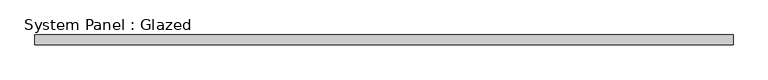
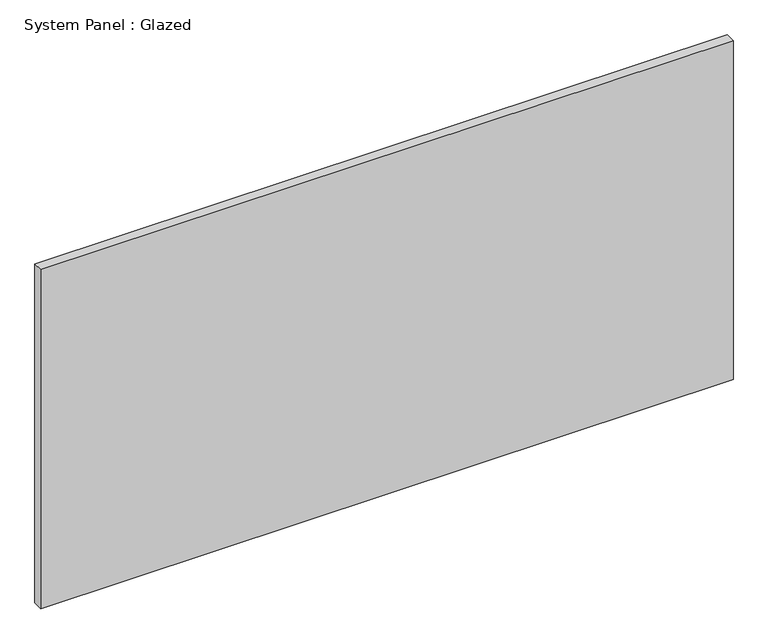
"""IFC4 building model written with IfcOpenShell, lengths in millimetres: plate geometry, System Panel : Glazed."""

from ifc_helpers import new_model, si_unit, origin, origin_with_axes, place, context, project, spatial, polyline, outline, extrude, source, transform, mapped, element, save


def system_panel_glazed_c1a1c740(model_context):
    return source(origin(), model_context, "Body", "SweptSolid", [
        extrude(outline(polyline([(882.65, 19.05), (-882.65, 19.05), (-882.65, 44.45), (882.65, 44.45), (882.65, 19.05)])), origin_with_axes(), (0.0, 0.0, 1.0), 914.4),
    ])


if __name__ == "__main__":
    model = new_model("IFC4")
    model_context = context("Model", 3, world=origin())
    ifc_project = project(units=[si_unit("LENGTHUNIT", "METRE", prefix="MILLI")], contexts=[model_context])
    site = spatial("IfcSite", under=ifc_project)
    building = spatial("IfcBuilding", under=site)
    placement = place(None, origin())
    system_panel_glazed_shape = system_panel_glazed_c1a1c740(model_context)
    element("IfcPlate", 1, ObjectType="System Panel : Glazed", at=placement, inside=building, context=model_context, shape_type="MappedRepresentation", body=[
        mapped(system_panel_glazed_shape, transform((0.0, 0.0, 0.0), x_axis=(1.0, 0.0, 0.0), y_axis=(0.0, 1.0, 0.0), z_axis=(0.0, 0.0, 1.0))),
    ])
    save(model, "model.ifc")

# Revit data of these elements
# Type "System Panel : Glazed"
#   Construction Type Id = "GSP4R"
#   Analytic Construction = "1/8 in Pilkington single glazing"
#   Visual Light Transmittance = 0.9
#   Solar Heat Gain Coefficient = 0.86
#   Heat Transfer Coefficient (U) = 6.7069 W/(m²·K)
# Element 1 (IfcPlate, "System Panel : Glazed")
#   Materials on its faces: "Glass"
# Materials
#   "Glass": class "Glass", colour RGB 0 128 192, transparency 0.75, Description = "Soda Lime Glass", Cost = 0
